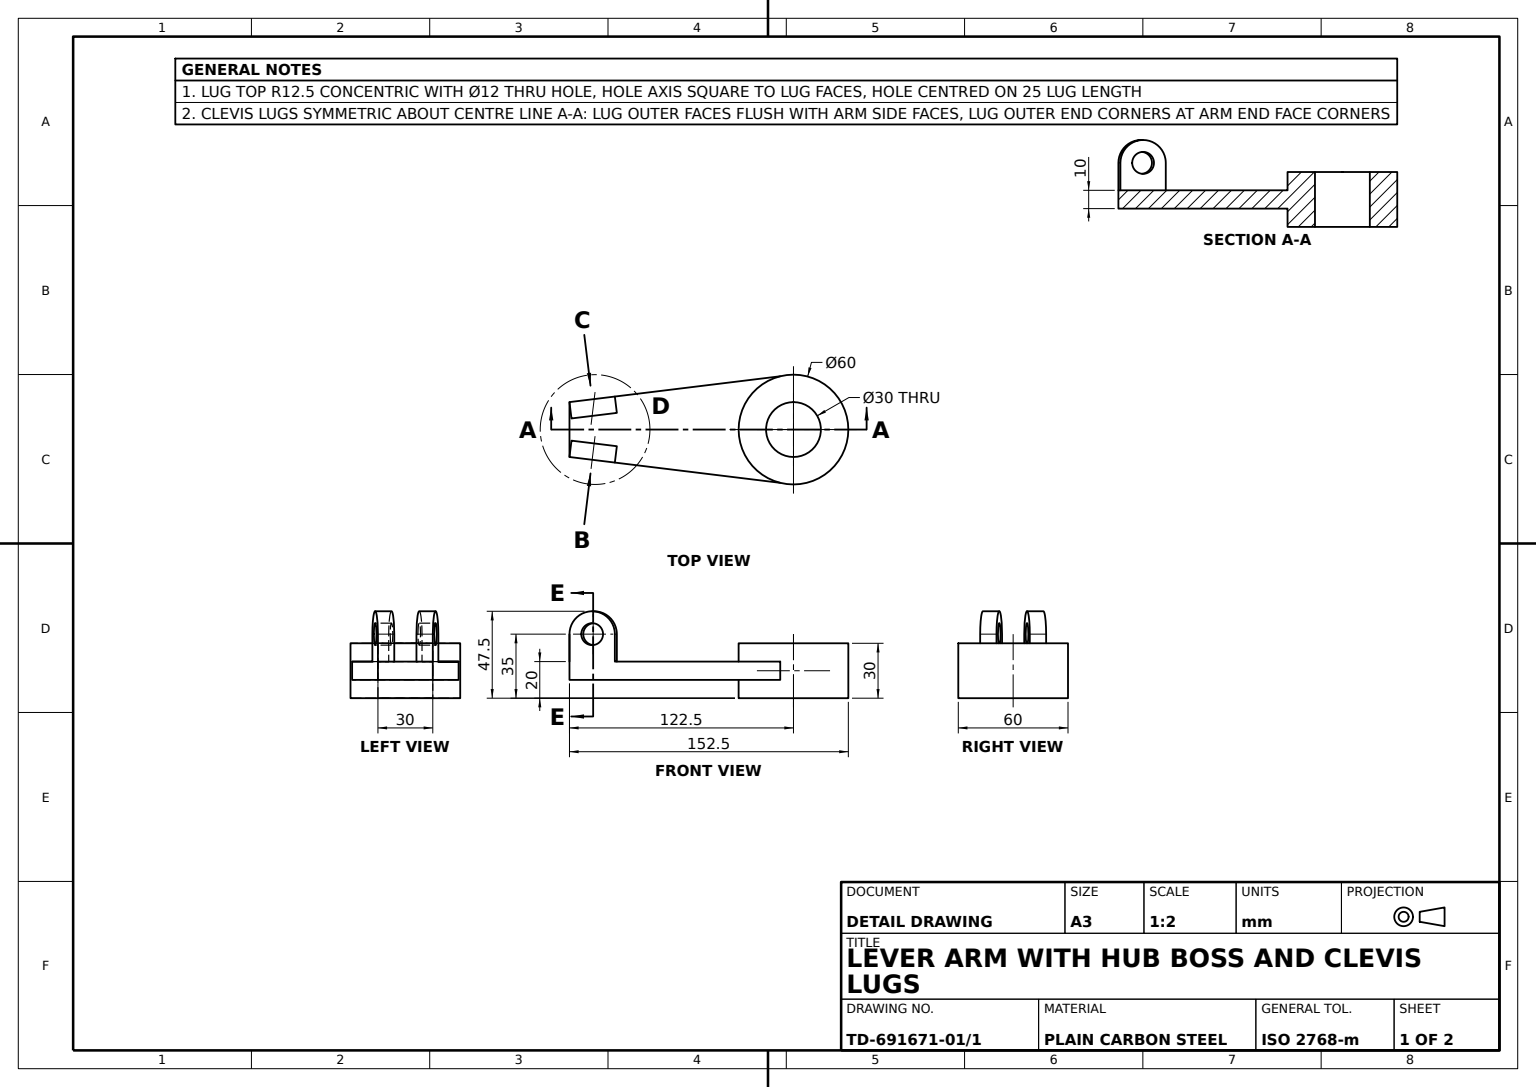
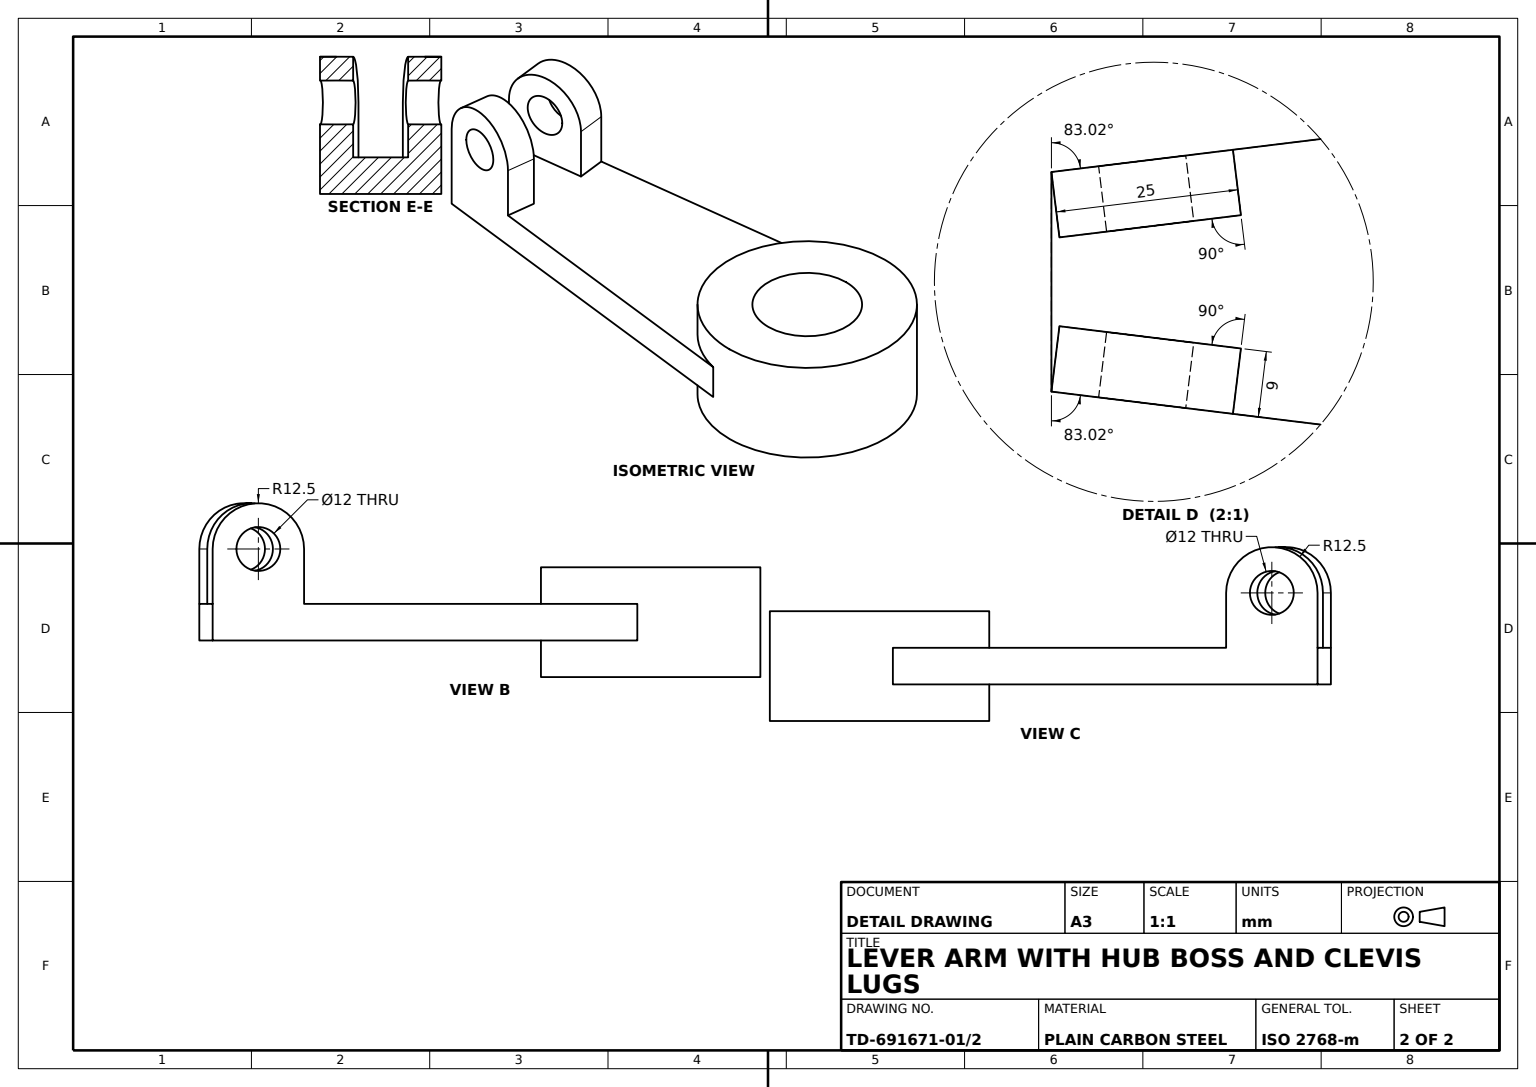
SolidWorks part; units mm, degrees
material "Plain Carbon Steel"
ref_plane "Front Plane" through (0, 0, 0) normal (0, 0, 1) x (1, 0, 0)
ref_plane "Top Plane" through (0, 0, 0) normal (0, 1, 0) x (1, 0, 0)
ref_plane "Right Plane" through (0, 0, 0) normal (1, 0, 0) x (0, 0, -1)
sketch "Hub Profile Sketch" plane through (0, 0, 0) normal (0, 1, 0) x (1, 0, 0)
  circle A0 centre (0, 0) radius 30
  dimension "D1" = 60
extrude "Hub Ø60" add sketch "Hub Profile Sketch" along normal blind 20
sketch "Arm Profile Sketch" plane through (0, 0, 0) normal (0, 1, 0) x (1, 0, 0)
  line L0 (0, 0) -> (-122.5, 0) construction
  line L1 (-122.5, 0) -> (-122.5, 15)
  line L2 (-122.5, 15) -> (0, 30)
  line L3 (-122.5, 0) -> (-122.5, -15)
  line L4 (-122.5, -15) -> (0, -30)
  circle A0 centre (0, 0) radius 30 construction
  circle A1 centre (0, 0) radius 30 construction
  arc A2 (0, 30) -> (0, -30) centre (0, 0) ccw
  dimension "D1" = 15
  dimension "D2" = 15
  dimension "D3" = 122.5
extrude "Lever Arm" add sketch "Arm Profile Sketch" along normal blind 10 contours L0 A2 L2 L1 | A2 L0 L3 L4
sketch "Hub Extension Sketch" plane through (0, 0, 0) normal (0, -1, 0) x (1, 0, 0)
  circle A0 centre (0, 0) radius 30
  dimension "D1" = 60
extrude "Hub Extension" add sketch "Hub Extension Sketch" along normal blind 20
sketch "Clevis Lug Sketch" plane through (-3.6192, 0, -29.5568) normal (-0.1215, 0, -0.9926) x (-0.9926, 0, 0.1215)
  line L0 (119.7687, 0) -> (119.7687, 25)
  line L2 (94.7687, 25) -> (94.7687, 0)
  line L3 (119.7687, 0) -> (3.6462, 0) construction
  line L4 (94.7687, 0) -> (119.7687, 0)
  arc A0 (119.7687, 25) -> (94.7687, 25) centre (107.2687, 25) ccw
  circle A1 centre (107.2687, 25) radius 6
  dimension "D3" = 12
  dimension "D1" = 25
  dimension "D2" = 25
extrude "Clevis Lug" add sketch "Clevis Lug Sketch" against normal blind 9
mirror "Clevis Lug Mirror" about plane through (0, 0, 0) normal (0, 0, 1) of bodies 106
sketch "Hub Recess Sketch" plane through (0, -20, 0) normal (0, -1, 0) x (-1, 0, 0)
  circle A0 centre (0, 0) radius 30
  dimension "D1" = 60
extrude "Hub Recess Cut" cut sketch "Hub Recess Sketch" against normal blind 10
sketch "Bore Sketch" plane through (0, -10, 0) normal (0, -1, 0) x (-1, 0, 0)
  circle A0 centre (0, 0) radius 15
  dimension "D1" = 30
extrude "Hub Bore Ø30" cut sketch "Bore Sketch" against normal blind 46
